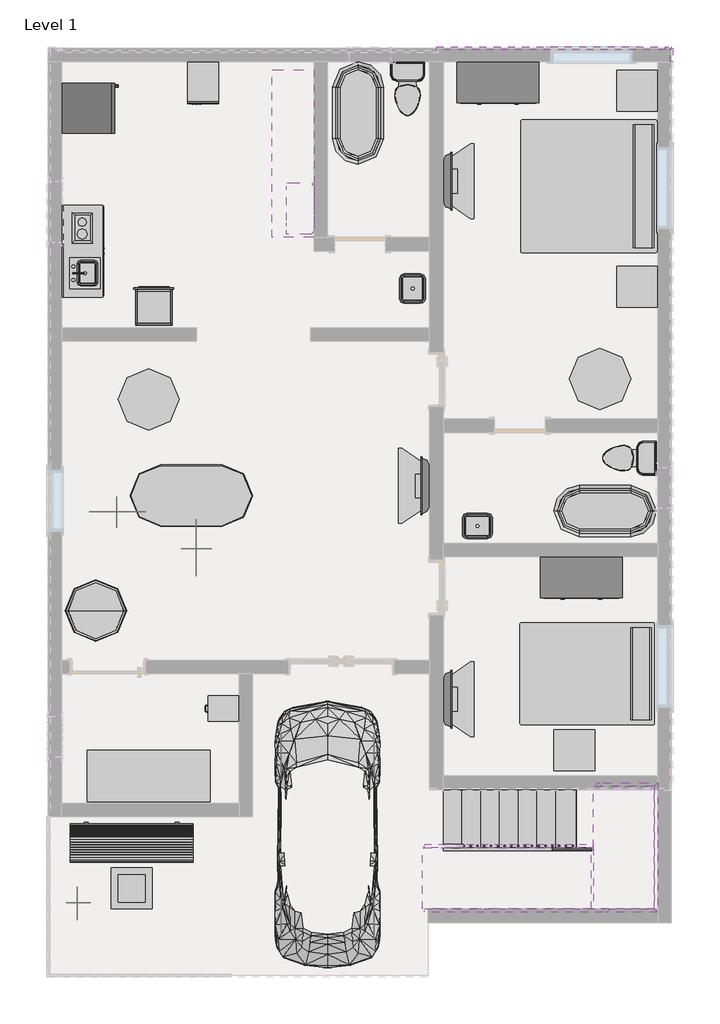
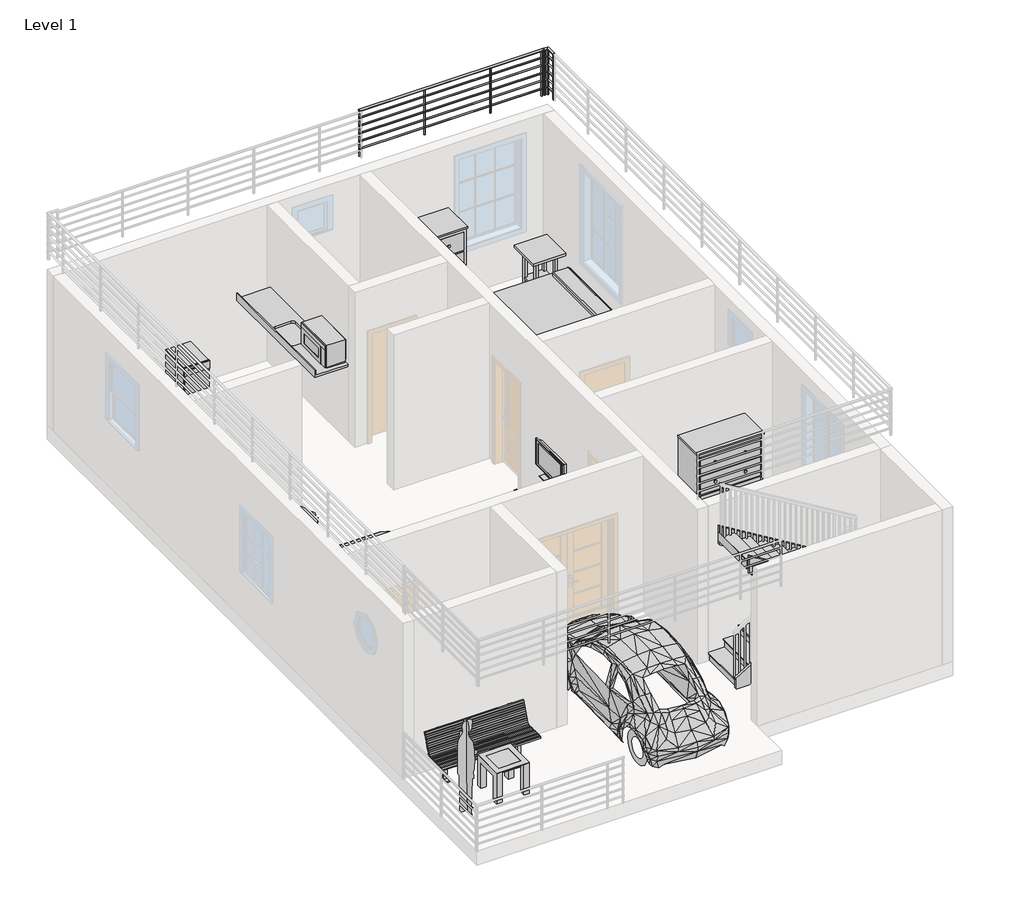
# One storey, part 4 of 4: 22 furniture elements, 10 proxies, 7 flow terminals, 7 members, 3 railings, 2 stair flights, 1 geographic element, 1 slab.
"""IFC4 building model written with IfcOpenShell, lengths in millimetres."""

from ifc_helpers import new_model, si_unit, point, frame, frame_2d, origin, place, context, project, spatial, polyline, circle_curve, trimmed, segment, composite_curve, outline, extrude, faceted_brep, transform, mapped, element, save
from components import proxy_7e1014cc, proxy_fe84b772, proxy_844211aa, proxy_8a8d5ab2, proxy_8b8c2dc4, rpc_beetle_rpc_beetle_3ce7ba48, rpc_female_69e001fa, rpc_male_28878092, proxy_a13a33b2, flow_terminal_871c2e40, flow_terminal_62a433f7, toilet_domestic_3d_toilet_domestic_3d_f7549cf7, toilet_domestic_3d_toilet_domestic_3d_183bbd19, flow_terminal_b374fae2, furniture_1fc5af50, furniture_e1791683, furniture_552c1472, counter_top_w_sink_hole_0600mm_depth_f226a61d, furniture_95afb093, furniture_9fa109b2, furniture_56245f3a, tv_stand_tv_stand_6ce107e5, furniture_b5c51a22, furniture_2c34a4f9, furniture_905aceb5, furniture_4bee3317, furniture_5bc9ed15, furniture_a5b052b6, furniture_c80d6d9c, geographic_element_235d1464, non_monolithic_landing_66cdc52a, stair_flight_35773103, stair_flight_b4d473f5

model = new_model("IFC4")

# Units and contexts
model_context = context("Model", 3, world=origin())
ifc_project = project(units=[si_unit("LENGTHUNIT", "METRE", prefix="MILLI")], contexts=[model_context])

# Site, building, storey
site = spatial("IfcSite", under=ifc_project)
building = spatial("IfcBuilding", under=site)
storey = spatial("IfcBuildingStorey", under=building, Name="Level 1", Elevation=0.0)

# Proxies
placement = place(None, origin())
proxy_shape = proxy_7e1014cc(model_context)
element("IfcBuildingElementProxy", 1, Name="18\" x 24\" x 34 1/2\"", ObjectType="18\" x 24\" x 34 1/2\"", at=placement, inside=storey, context=model_context, shape_type="MappedRepresentation", body=[
    mapped(proxy_shape, transform((-12417.3564253, 14333.684711, 0.0), x_axis=(1.0, 0.0, 0.0), y_axis=(0.0, 1.0, 0.0), z_axis=(0.0, 0.0, 1.0))),
])
proxy_2_shape = proxy_fe84b772(model_context)
element("IfcBuildingElementProxy", 2, Name="Cook Top-2 Unit : 12\" x 18\"", ObjectType="Cook Top-2 Unit : 12\" x 18\"", at=placement, inside=storey, context=model_context, shape_type="MappedRepresentation", body=[
    mapped(proxy_2_shape, transform((-13838.4389568, 12458.6590714, 0.0), x_axis=(-1.0000000000000002, 0.0, 0.0), y_axis=(0.0, -1.0000000000000002, 0.0), z_axis=(0.0, 0.0, 1.0))),
])
proxy_3_shape = proxy_844211aa(model_context)
element("IfcBuildingElementProxy", 3, Name="Kitchenette - Small : 54\"", ObjectType="Kitchenette - Small : 54\"", at=placement, inside=storey, context=model_context, shape_type="MappedRepresentation", body=[
    mapped(proxy_3_shape, transform((-14219.4389568, 12066.7965709, 0.0), x_axis=(0.0, 1.0000000000000002, 0.0), y_axis=(-1.0000000000000002, 0.0, 0.0), z_axis=(0.0, 0.0, 1.0))),
])
proxy_4_shape = proxy_8a8d5ab2(model_context)
element("IfcBuildingElementProxy", 4, Name="Microwave : 30\" x 16\" x 18\"", ObjectType="Microwave : 30\" x 16\" x 18\"", at=placement, inside=storey, context=model_context, shape_type="MappedRepresentation", body=[
    mapped(proxy_4_shape, transform((-10310.358451, 13220.8271532, 609.6), x_axis=(0.0, -1.0000000000000004, 0.0), y_axis=(1.0000000000000004, 0.0, 0.0), z_axis=(0.0, 0.0, 1.0))),
])
proxy_5_shape = proxy_8b8c2dc4(model_context)
element("IfcBuildingElementProxy", 5, Name="Oven Double-Built-in : 21 1/2\" x 39 1/4\" x 21\"", ObjectType="Oven Double-Built-in : 21 1/2\" x 39 1/4\" x 21\"", at=placement, inside=storey, context=model_context, shape_type="MappedRepresentation", body=[
    mapped(proxy_5_shape, transform((-12883.0138841, 11388.4001348, 0.0), x_axis=(-1.0000000000000004, 0.0, 0.0), y_axis=(0.0, -1.0000000000000004, 0.0), z_axis=(0.0, 0.0, 1.0))),
])
rpc_beetle_rpc_beetle_shape = rpc_beetle_rpc_beetle_3ce7ba48(model_context)
element("IfcBuildingElementProxy", 6, Name="RPC Beetle : RPC Beetle", ObjectType="RPC Beetle : RPC Beetle", at=placement, inside=storey, context=model_context, shape_type="MappedRepresentation", body=[
    mapped(rpc_beetle_rpc_beetle_shape, transform((-10257.0389568, 2154.1342758, 0.0), x_axis=(1.0, 0.0, 0.0), y_axis=(0.0, 1.0, 0.0), z_axis=(0.0, 0.0, 1.0))),
])
rpc_female_shape = rpc_female_69e001fa(model_context)
element("IfcBuildingElementProxy", 7, Name="RPC Female", ObjectType="RPC Female", at=placement, inside=storey, context=model_context, shape_type="MappedRepresentation", body=[
    mapped(rpc_female_shape, transform((-13241.5389568, 8191.0885751, 0.0), x_axis=(0.0, 1.0000000000000002, 0.0), y_axis=(-1.0000000000000002, 0.0, 0.0), z_axis=(0.0, 0.0, 1.0))),
])
element("IfcBuildingElementProxy", 8, Name="RPC Female", ObjectType="RPC Female", at=placement, inside=storey, context=model_context, shape_type="MappedRepresentation", body=[
    mapped(rpc_female_shape, transform((-12212.8389568, 7811.9842758, 0.0), x_axis=(-1.0000000000000002, 0.0, 0.0), y_axis=(0.0, -1.0000000000000002, 0.0), z_axis=(0.0, 0.0, 1.0))),
])
rpc_male_shape = rpc_male_28878092(model_context)
element("IfcBuildingElementProxy", 9, Name="RPC Male", ObjectType="RPC Male", at=placement, inside=storey, context=model_context, shape_type="MappedRepresentation", body=[
    mapped(rpc_male_shape, transform((-13990.8389568, 2357.3342758, 0.0), x_axis=(0.0, 1.0000000000000002, 0.0), y_axis=(-1.0000000000000002, 0.0, 0.0), z_axis=(0.0, 0.0, 1.0))),
])
proxy_6_shape = proxy_a13a33b2(model_context)
element("IfcBuildingElementProxy", 10, Name="Refrigerator : 30\" x 32\" RH", ObjectType="Refrigerator : 30\" x 32\" RH", at=placement, inside=storey, context=model_context, shape_type="MappedRepresentation", body=[
    mapped(proxy_6_shape, transform((-13846.3764568, 14211.5853043, 0.0), x_axis=(0.0, 1.0000000000000009, 0.0), y_axis=(-1.0000000000000009, 0.0, 0.0), z_axis=(0.0, 0.0, 1.0))),
])

# Flow terminals
flow_terminal_shape = flow_terminal_871c2e40(model_context)
element("IfcFlowTerminal", 11, ObjectType="Sink Kitchen-Island : 18\" x 18\"", at=placement, inside=storey, context=model_context, shape_type="MappedRepresentation", body=[
    mapped(flow_terminal_shape, transform((-13874.1935557, 11739.6450353, 0.0), x_axis=(0.0, 1.0000000000000002, 0.0), y_axis=(-1.0000000000000002, 0.0, 0.0), z_axis=(0.0, 0.0, 1.0))),
])
flow_terminal_2_shape = flow_terminal_62a433f7(model_context)
element("IfcFlowTerminal", 12, ObjectType="Sink Vanity-Square : 20\" x 18\"", at=placement, inside=storey, context=model_context, shape_type="MappedRepresentation", body=[
    mapped(flow_terminal_2_shape, transform((-8006.1497162, 7934.9796769, 609.6), x_axis=(-1.0000000000000002, 0.0, 0.0), y_axis=(0.0, -1.0000000000000002, 0.0), z_axis=(0.0, 0.0, 1.0))),
])
element("IfcFlowTerminal", 13, ObjectType="Sink Vanity-Square : 20\" x 18\"", at=placement, inside=storey, context=model_context, shape_type="MappedRepresentation", body=[
    mapped(flow_terminal_2_shape, transform((-8938.5843579, 11542.4235164, 609.6), x_axis=(0.0, -1.0, 0.0), y_axis=(1.0, 0.0, 0.0), z_axis=(0.0, 0.0, 1.0))),
])
toilet_domestic_3d_toilet_domestic_3d_shape = toilet_domestic_3d_toilet_domestic_3d_f7549cf7(model_context)
toilet_domestic_3d_toilet_domestic_3d_2_shape = toilet_domestic_3d_toilet_domestic_3d_183bbd19(model_context)
element("IfcFlowTerminal", 14, ObjectType="Toilet-Domestic-3D : Toilet-Domestic-3D", at=placement, inside=storey, context=model_context, shape_type="MappedRepresentation", body=[
    mapped(toilet_domestic_3d_toilet_domestic_3d_shape, transform((-9063.2389568, 14410.2382485, 0.0), x_axis=(1.0000000000000002, 0.0, 0.0), y_axis=(0.0, 1.0000000000000002, 0.0), z_axis=(0.0, 0.0, 1.0))),
    mapped(toilet_domestic_3d_toilet_domestic_3d_2_shape, transform((-9063.2389568, 14410.2382485, 0.0), x_axis=(1.0000000000000002, 0.0, 0.0), y_axis=(0.0, 1.0000000000000002, 0.0), z_axis=(0.0, 0.0, 1.0))),
])
element("IfcFlowTerminal", 15, ObjectType="Toilet-Domestic-3D : Toilet-Domestic-3D", at=placement, inside=storey, context=model_context, shape_type="MappedRepresentation", body=[
    mapped(toilet_domestic_3d_toilet_domestic_3d_shape, transform((-5849.5349842, 8999.4342758, 0.0), x_axis=(0.0, -1.0000000000000004, 0.0), y_axis=(1.0000000000000004, 0.0, 0.0), z_axis=(0.0, 0.0, 1.0))),
    mapped(toilet_domestic_3d_toilet_domestic_3d_2_shape, transform((-5849.5349842, 8999.4342758, 0.0), x_axis=(0.0, -1.0000000000000004, 0.0), y_axis=(1.0000000000000004, 0.0, 0.0), z_axis=(0.0, 0.0, 1.0))),
])
flow_terminal_3_shape = flow_terminal_b374fae2(model_context)
element("IfcFlowTerminal", 16, ObjectType="Tub-Free Standing-3D : 30\" x 60\"", at=placement, inside=storey, context=model_context, shape_type="MappedRepresentation", body=[
    mapped(flow_terminal_3_shape, transform((-9799.8389568, 14142.9342758, 0.0), x_axis=(1.0, 0.0, 0.0), y_axis=(0.0, 1.0, 0.0), z_axis=(0.0, 0.0, 1.0))),
])
element("IfcFlowTerminal", 17, ObjectType="Tub-Free Standing-3D : 30\" x 60\"", at=placement, inside=storey, context=model_context, shape_type="MappedRepresentation", body=[
    mapped(flow_terminal_3_shape, transform((-6116.8389568, 8212.0342758, 0.0), x_axis=(0.0, -1.0000000000000004, 0.0), y_axis=(1.0000000000000004, 0.0, 0.0), z_axis=(0.0, 0.0, 1.0))),
])

# Furniture
furniture_shape = furniture_1fc5af50(model_context)
element("IfcFurniture", 18, ObjectType="Bed-Standard.0001 : King 78\" x 80\"", at=placement, inside=storey, context=model_context, shape_type="MappedRepresentation", body=[
    mapped(furniture_shape, transform((-6312.5438748, 13322.2228004, 0.0), x_axis=(0.0, -1.0, 0.0), y_axis=(1.0, 0.0, 0.0), z_axis=(0.0, 0.0, 1.0))),
])
furniture_2_shape = furniture_e1791683(model_context)
element("IfcFurniture", 19, ObjectType="Bed-Standard.0001 : Queen 60\" x 79\"", at=placement, inside=storey, context=model_context, shape_type="MappedRepresentation", body=[
    mapped(furniture_2_shape, transform((-6337.9438748, 6057.8228004, 0.0), x_axis=(0.0, -1.0, 0.0), y_axis=(1.0, 0.0, 0.0), z_axis=(0.0, 0.0, 1.0))),
])
furniture_3_shape = furniture_552c1472(model_context)
element("IfcFurniture", 20, ObjectType="Cabinet-File 3 Drawer.0001 : 15\" x 18\"", at=placement, inside=storey, context=model_context, shape_type="MappedRepresentation", body=[
    mapped(furniture_3_shape, transform((-11664.3046567, 5137.7378288, 0.0), x_axis=(0.0, -1.0000000000000004, 0.0), y_axis=(1.0000000000000004, 0.0, 0.0), z_axis=(0.0, 0.0, 1.0))),
])
counter_top_w_sink_hole_0600mm_depth_shape = counter_top_w_sink_hole_0600mm_depth_f226a61d(model_context)
element("IfcFurniture", 21, ObjectType="Counter Top w Sink Hole : 0600mm Depth", at=placement, inside=storey, context=model_context, shape_type="MappedRepresentation", body=[
    mapped(counter_top_w_sink_hole_0600mm_depth_shape, transform((-11084.9202068, 13489.1965709, 609.6), x_axis=(0.0, 1.0, 0.0), y_axis=(-1.0, 0.0, 0.0), z_axis=(0.0, 0.0, 1.0))),
])
furniture_4_shape = furniture_95afb093(model_context)
element("IfcFurniture", 22, ObjectType="Counter Top w Sink Hole : 24\" Depth", at=placement, inside=storey, context=model_context, shape_type="MappedRepresentation", body=[
    mapped(furniture_4_shape, transform((-14219.4389568, 12600.1965709, 0.0), x_axis=(0.0, 1.0000000000000002, 0.0), y_axis=(-1.0000000000000002, 0.0, 0.0), z_axis=(0.0, 0.0, 1.0))),
])
furniture_5_shape = furniture_9fa109b2(model_context)
element("IfcFurniture", 23, ObjectType="Dresser : 48\" x 72\" x 24\"", at=placement, inside=storey, context=model_context, shape_type="MappedRepresentation", body=[
    mapped(furniture_5_shape, transform((-7447.845697, 14963.2972299, 0.0), x_axis=(1.0000000000000004, 0.0, 0.0), y_axis=(0.0, 1.0000000000000004, 0.0), z_axis=(0.0, 0.0, 1.0))),
])
element("IfcFurniture", 24, ObjectType="Dresser.0001 : 48\" x 72\" x 24\"", at=placement, inside=storey, context=model_context, shape_type="MappedRepresentation", body=[
    mapped(furniture_5_shape, transform((-6203.245697, 7584.5972299, 0.0), x_axis=(1.0, 0.0, 0.0), y_axis=(0.0, 1.0, 0.0), z_axis=(0.0, 0.0, 1.0))),
])
furniture_6_shape = furniture_56245f3a(model_context)
element("IfcFurniture", 25, ObjectType="TV - Flat Screen : 32\"", at=placement, inside=storey, context=model_context, shape_type="MappedRepresentation", body=[
    mapped(furniture_6_shape, transform((-8471.3003332, 5409.27879, 914.4), x_axis=(0.0, 1.0, 0.0), y_axis=(-1.0, 0.0, 0.0), z_axis=(0.0, 0.0, 1.0))),
])
element("IfcFurniture", 26, ObjectType="TV - Flat Screen : 32\"", at=placement, inside=storey, context=model_context, shape_type="MappedRepresentation", body=[
    mapped(furniture_6_shape, transform((-8471.3003332, 13130.87879, 914.4), x_axis=(0.0, 1.0, 0.0), y_axis=(-1.0, 0.0, 0.0), z_axis=(0.0, 0.0, 1.0))),
])
element("IfcFurniture", 27, ObjectType="TV - Flat Screen : 32\"", at=placement, inside=storey, context=model_context, shape_type="MappedRepresentation", body=[
    mapped(furniture_6_shape, transform((-8797.5381048, 8582.222, 914.4), x_axis=(0.0, -1.0000000000000004, 0.0), y_axis=(1.0000000000000004, 0.0, 0.0), z_axis=(0.0, 0.0, 1.0))),
])
tv_stand_tv_stand_shape = tv_stand_tv_stand_6ce107e5(model_context)
element("IfcFurniture", 28, ObjectType="TV Stand : TV Stand", at=placement, inside=storey, context=model_context, shape_type="MappedRepresentation", body=[
    mapped(tv_stand_tv_stand_shape, transform((-8529.8389568, 13001.7462738, 0.0), x_axis=(0.0, 1.0000000000000002, 0.0), y_axis=(-1.0000000000000002, 0.0, 0.0), z_axis=(0.0, 0.0, 1.0))),
])
element("IfcFurniture", 29, ObjectType="TV Stand : TV Stand", at=placement, inside=storey, context=model_context, shape_type="MappedRepresentation", body=[
    mapped(tv_stand_tv_stand_shape, transform((-8529.8389568, 5280.1462738, 0.0), x_axis=(0.0, 1.0000000000000002, 0.0), y_axis=(-1.0000000000000002, 0.0, 0.0), z_axis=(0.0, 0.0, 1.0))),
])
element("IfcFurniture", 30, ObjectType="TV Stand : TV Stand", at=placement, inside=storey, context=model_context, shape_type="MappedRepresentation", body=[
    mapped(tv_stand_tv_stand_shape, transform((-8738.9994812, 8711.3545162, 0.0), x_axis=(0.0, -1.0000000000000007, 0.0), y_axis=(1.0000000000000007, 0.0, 0.0), z_axis=(0.0, 0.0, 1.0))),
])
furniture_7_shape = furniture_b5c51a22(model_context)
element("IfcFurniture", 31, ObjectType="Table-Coffee : 24\" x 24\" x 24\"", at=placement, inside=storey, context=model_context, shape_type="MappedRepresentation", body=[
    mapped(furniture_7_shape, transform((-13196.3047235, 2490.723198, 0.0), x_axis=(1.0, 0.0, 0.0), y_axis=(0.0, 1.0, 0.0), z_axis=(0.0, 0.0, 1.0))),
])
furniture_8_shape = furniture_2c34a4f9(model_context)
element("IfcFurniture", 32, ObjectType="Table-Dining Oval : 36\" x 72\"", at=placement, inside=storey, context=model_context, shape_type="MappedRepresentation", body=[
    mapped(furniture_8_shape, transform((-12690.8586289, 8082.5359152, 0.0), x_axis=(-1.0, 0.0, 0.0), y_axis=(0.0, -1.0, 0.0), z_axis=(0.0, 0.0, 1.0))),
])
furniture_9_shape = furniture_905aceb5(model_context)
element("IfcFurniture", 33, ObjectType="Table-Dining Round w Chairs : 36\" Diameter", at=placement, inside=storey, context=model_context, shape_type="MappedRepresentation", body=[
    mapped(furniture_9_shape, transform((-13027.720924, 10060.6129644, 0.0), x_axis=(1.0, 0.0, 0.0), y_axis=(0.0, 1.0, 0.0), z_axis=(0.0, 0.0, 1.0))),
])
furniture_10_shape = furniture_4bee3317(model_context)
element("IfcFurniture", 34, ObjectType="Table-Ellipse : 72\" x 36\"", at=placement, inside=storey, context=model_context, shape_type="MappedRepresentation", body=[
    mapped(furniture_10_shape, transform((-6193.0389568, 10180.5342758, 0.0), x_axis=(1.0, 0.0, 0.0), y_axis=(0.0, 1.0, 0.0), z_axis=(0.0, 0.0, 1.0))),
])
furniture_11_shape = furniture_5bc9ed15(model_context)
element("IfcFurniture", 35, ObjectType="Table-Night Stand : 24\" x 24\" x 30\"", at=placement, inside=storey, context=model_context, shape_type="MappedRepresentation", body=[
    mapped(furniture_11_shape, transform((-5942.7725871, 14168.3342758, 0.0), x_axis=(1.0, 0.0, 0.0), y_axis=(0.0, 1.0, 0.0), z_axis=(0.0, 0.0, 1.0))),
])
element("IfcFurniture", 36, ObjectType="Table-Night Stand : 24\" x 24\" x 30\"", at=placement, inside=storey, context=model_context, shape_type="MappedRepresentation", body=[
    mapped(furniture_11_shape, transform((-5942.7725871, 11247.3342758, 0.0), x_axis=(1.0, 0.0, 0.0), y_axis=(0.0, 1.0, 0.0), z_axis=(0.0, 0.0, 1.0))),
])
element("IfcFurniture", 37, ObjectType="Table-Night Stand : 24\" x 24\" x 30\"", at=placement, inside=storey, context=model_context, shape_type="MappedRepresentation", body=[
    mapped(furniture_11_shape, transform((-6882.5725871, 4338.5342758, 0.0), x_axis=(1.0, 0.0, 0.0), y_axis=(0.0, 1.0, 0.0), z_axis=(0.0, 0.0, 1.0))),
])
furniture_12_shape = furniture_a5b052b6(model_context)
element("IfcFurniture", 38, ObjectType="Table-Rectangular : 72\" x 30\"", at=placement, inside=storey, context=model_context, shape_type="MappedRepresentation", body=[
    mapped(furniture_12_shape, transform((-12924.0389568, 4262.3342758, 0.0), x_axis=(1.0, 0.0, 0.0), y_axis=(0.0, 1.0, 0.0), z_axis=(0.0, 0.0, 1.0))),
])
furniture_13_shape = furniture_c80d6d9c(model_context)
element("IfcFurniture", 39, ObjectType="Table-Round : 36\" Diameter", at=placement, inside=storey, context=model_context, shape_type="MappedRepresentation", body=[
    mapped(furniture_13_shape, transform((-13711.4389568, 6726.1342758, 0.0), x_axis=(1.0, 0.0, 0.0), y_axis=(0.0, 1.0, 0.0), z_axis=(0.0, 0.0, 1.0))),
])

# Geographic element
geographic_element_shape = geographic_element_235d1464(model_context)
element("IfcGeographicElement", 40, ObjectType="Park Bench : 72\"", at=placement, inside=storey, context=model_context, shape_type="MappedRepresentation", body=[
    mapped(geographic_element_shape, transform((-13178.0389568, 3297.1342758, 0.0), x_axis=(1.0, 0.0, 0.0), y_axis=(0.0, 1.0, 0.0), z_axis=(0.0, 0.0, 1.0))),
])

# Members
element("IfcMember", 41, ObjectType="Stringer - 2\" Width", at=placement, inside=storey, context=model_context, shape_type="SweptSolid", body=[
    extrude(outline(polyline([(212.114512, -8529.8389568), (0.0, -8529.8389568), (0.0, -8291.753445), (1295.4, -6154.343445), (1600.2, -6239.4979015), (212.114512, -8529.8389568)])), frame((0.0, 4109.9342758, 0.0), z_axis=(0.0, 1.0, 0.0), x_axis=(0.0, 0.0, 1.0)), (0.0, 0.0, 1.0), 50.8),
])
element("IfcMember", 42, ObjectType="Stringer - 2\" Width", at=placement, inside=storey, context=model_context, shape_type="Brep", body=[
    faceted_brep([(-8529.8389568, 3144.7342758, 0.0), (-8529.8389568, 3195.5342758, 0.0), (-8291.753445, 3195.5342758, 0.0), (-8291.753445, 3144.7342758, 0.0), (-8529.8389568, 3144.7342758, 212.114512), (-8529.8389568, 3195.5342758, 212.114512), (-6294.6389568, 3144.7342758, 1566.7811786), (-6294.6389568, 3195.5342758, 1566.7811786), (-6294.6389568, 3195.5342758, 1379.7057504), (-6294.6389568, 3195.5342758, 1210.3724171), (-6294.6389568, 3144.7342758, 1210.3724171)], [[[0, 1, 2, 3]], [[4, 5, 1, 0]], [[5, 4, 6, 7]], [[1, 5, 7, 8, 9, 2]], [[4, 0, 3, 10, 6]], [[2, 9, 10, 3]], [[6, 10, 9, 8, 7]]]),
])
element("IfcMember", 43, ObjectType="Stringer - 2\" Width", at=placement, inside=storey, context=model_context, shape_type="SweptSolid", body=[
    extrude(outline(polyline([(1295.4, -6155.5344686), (1600.2, -6070.3800121), (3260.114512, -8809.2389568), (2903.7057504, -8809.2389568), (1295.4, -6155.5344686)])), frame((0.0, 2230.3342758, 0.0), z_axis=(0.0, 1.0, 0.0), x_axis=(0.0, 0.0, 1.0)), (0.0, 0.0, 1.0), 50.8),
])
element("IfcMember", 44, ObjectType="Stringer - 2\" Width", at=placement, inside=storey, context=model_context, shape_type="Brep", body=[
    faceted_brep([(-8809.2389568, 3246.3342758, 3260.114512), (-8809.2389568, 3246.3342758, 2903.7057504), (-8809.2389568, 3195.5342758, 2903.7057504), (-8809.2389568, 3195.5342758, 3260.114512), (-6294.6389568, 3195.5342758, 1736.114512), (-6294.6389568, 3246.3342758, 1736.114512), (-6294.6389568, 3195.5342758, 1379.7057504), (-6294.6389568, 3195.5342758, 1566.7811786), (-6294.6389568, 3246.3342758, 1379.7057504)], [[[0, 1, 2, 3]], [[4, 5, 0, 3]], [[6, 7, 4, 3, 2]], [[8, 6, 2, 1]], [[5, 8, 1, 0]], [[5, 4, 7, 6, 8]]]),
])
element("IfcMember", 45, ObjectType="Stringer - 2\" Width", at=placement, inside=storey, context=model_context, shape_type="Brep", body=[
    faceted_brep([(-6070.3800121, 2281.1342758, 1600.2), (-6070.3800121, 2230.3342758, 1600.2), (-5329.4389568, 2230.3342758, 1600.2), (-5380.2389568, 2281.1342758, 1600.2), (-6155.5344686, 2281.1342758, 1295.4), (-5380.2389568, 2281.1342758, 1295.4), (-6155.5344686, 2230.3342758, 1295.4), (-5329.4389568, 2230.3342758, 1295.4)], [[[0, 1, 2, 3]], [[4, 0, 3, 5]], [[6, 4, 5, 7]], [[1, 6, 7, 2]], [[1, 0, 4, 6]], [[2, 7, 5, 3]]]),
])
element("IfcMember", 46, ObjectType="Stringer - 2\" Width", at=placement, inside=storey, context=model_context, shape_type="SweptSolid", body=[
    extrude(outline(polyline([(-5329.4389568, 2230.3342758), (-5380.2389568, 2281.1342758), (-5380.2389568, 4109.9342758), (-5329.4389568, 4160.7342758), (-5329.4389568, 2230.3342758)])), frame((0.0, 0.0, 1295.4), z_axis=(0.0, 0.0, 1.0), x_axis=(1.0, 0.0, 0.0)), (0.0, 0.0, 1.0), 304.8),
])
element("IfcMember", 47, ObjectType="Stringer - 2\" Width", at=placement, inside=storey, context=model_context, shape_type="Brep", body=[
    faceted_brep([(-5380.2389568, 4109.9342758, 1600.2), (-5329.4389568, 4160.7342758, 1600.2), (-6239.4979015, 4160.7342758, 1600.2), (-6239.4979015, 4109.9342758, 1600.2), (-5380.2389568, 4109.9342758, 1295.4), (-6154.343445, 4109.9342758, 1295.4), (-5329.4389568, 4160.7342758, 1295.4), (-6154.343445, 4160.7342758, 1295.4)], [[[0, 1, 2, 3]], [[4, 0, 3, 5]], [[6, 4, 5, 7]], [[1, 6, 7, 2]], [[1, 0, 4, 6]], [[2, 7, 5, 3]]]),
])

# Railings
element("IfcRailing", 48, ObjectType="Handrail - Pipe", at=placement, inside=storey, context=model_context, shape_type="SweptSolid", body=[
    extrude(outline(composite_curve([segment(trimmed(circle_curve(frame_2d((4146.55, -5126.2389568)), 19.05), [point((4146.55, -5107.1889568))], [point((4146.55, -5145.2889568))], False, "CARTESIAN"), True, "CONTINUOUS"), segment(trimmed(circle_curve(frame_2d((4146.55, -5126.2389568)), 19.05), [point((4146.55, -5145.2889568))], [point((4146.55, -5107.1889568))], False, "CARTESIAN"), True, "CONTINUOUS")], self_intersect=False)), frame((0.0, 14904.9342758, 0.0), z_axis=(0.0, 1.0, 0.0), x_axis=(0.0, 0.0, 1.0)), (0.0, 0.0, 1.0), 203.2),
    extrude(outline(composite_curve([segment(trimmed(circle_curve(frame_2d((4000.5, -5126.2389568)), 12.7), [point((4000.5, -5138.9389568))], [point((4000.5, -5113.5389568))], False, "CARTESIAN"), True, "CONTINUOUS"), segment(trimmed(circle_curve(frame_2d((4000.5, -5126.2389568)), 12.7), [point((4000.5, -5113.5389568))], [point((4000.5, -5138.9389568))], False, "CARTESIAN"), True, "CONTINUOUS")], self_intersect=False)), frame((0.0, 14904.9342758, 0.0), z_axis=(0.0, 1.0, 0.0), x_axis=(0.0, 0.0, 1.0)), (0.0, 0.0, 1.0), 203.2),
    extrude(outline(composite_curve([segment(trimmed(circle_curve(frame_2d((3848.1, -5126.2389568)), 12.7), [point((3848.1, -5138.9389568))], [point((3848.1, -5113.5389568))], False, "CARTESIAN"), True, "CONTINUOUS"), segment(trimmed(circle_curve(frame_2d((3848.1, -5126.2389568)), 12.7), [point((3848.1, -5113.5389568))], [point((3848.1, -5138.9389568))], False, "CARTESIAN"), True, "CONTINUOUS")], self_intersect=False)), frame((0.0, 14904.9342758, 0.0), z_axis=(0.0, 1.0, 0.0), x_axis=(0.0, 0.0, 1.0)), (0.0, 0.0, 1.0), 203.2),
    extrude(outline(composite_curve([segment(trimmed(circle_curve(frame_2d((3695.7, -5126.2389568)), 12.7), [point((3695.7, -5138.9389568))], [point((3695.7, -5113.5389568))], False, "CARTESIAN"), True, "CONTINUOUS"), segment(trimmed(circle_curve(frame_2d((3695.7, -5126.2389568)), 12.7), [point((3695.7, -5113.5389568))], [point((3695.7, -5138.9389568))], False, "CARTESIAN"), True, "CONTINUOUS")], self_intersect=False)), frame((0.0, 14904.9342758, 0.0), z_axis=(0.0, 1.0, 0.0), x_axis=(0.0, 0.0, 1.0)), (0.0, 0.0, 1.0), 203.2),
    extrude(outline(composite_curve([segment(trimmed(circle_curve(frame_2d((3543.3, -5126.2389568)), 12.7), [point((3543.3, -5138.9389568))], [point((3543.3, -5113.5389568))], False, "CARTESIAN"), True, "CONTINUOUS"), segment(trimmed(circle_curve(frame_2d((3543.3, -5126.2389568)), 12.7), [point((3543.3, -5113.5389568))], [point((3543.3, -5138.9389568))], False, "CARTESIAN"), True, "CONTINUOUS")], self_intersect=False)), frame((0.0, 14904.9342758, 0.0), z_axis=(0.0, 1.0, 0.0), x_axis=(0.0, 0.0, 1.0)), (0.0, 0.0, 1.0), 203.2),
    extrude(outline(composite_curve([segment(trimmed(circle_curve(frame_2d((3390.9, -5126.2389568)), 12.7), [point((3390.9, -5138.9389568))], [point((3390.9, -5113.5389568))], False, "CARTESIAN"), True, "CONTINUOUS"), segment(trimmed(circle_curve(frame_2d((3390.9, -5126.2389568)), 12.7), [point((3390.9, -5113.5389568))], [point((3390.9, -5138.9389568))], False, "CARTESIAN"), True, "CONTINUOUS")], self_intersect=False)), frame((0.0, 14904.9342758, 0.0), z_axis=(0.0, 1.0, 0.0), x_axis=(0.0, 0.0, 1.0)), (0.0, 0.0, 1.0), 203.2),
    extrude(outline(composite_curve([segment(trimmed(circle_curve(frame_2d((-5126.2389568, 15095.4342758)), 12.7), [point((-5138.9389568, 15095.4342758))], [point((-5113.5389568, 15095.4342758))], False, "CARTESIAN"), True, "CONTINUOUS"), segment(trimmed(circle_curve(frame_2d((-5126.2389568, 15095.4342758)), 12.7), [point((-5113.5389568, 15095.4342758))], [point((-5138.9389568, 15095.4342758))], False, "CARTESIAN"), True, "CONTINUOUS")], self_intersect=False)), frame((0.0, 0.0, 3251.2), z_axis=(0.0, 0.0, 1.0), x_axis=(1.0, 0.0, 0.0)), (0.0, 0.0, 1.0), 876.3),
    extrude(outline(composite_curve([segment(trimmed(circle_curve(frame_2d((-5126.2389568, 14917.6342758)), 12.7), [point((-5138.9389568, 14917.6342758))], [point((-5113.5389568, 14917.6342758))], False, "CARTESIAN"), True, "CONTINUOUS"), segment(trimmed(circle_curve(frame_2d((-5126.2389568, 14917.6342758)), 12.7), [point((-5113.5389568, 14917.6342758))], [point((-5138.9389568, 14917.6342758))], False, "CARTESIAN"), True, "CONTINUOUS")], self_intersect=False)), frame((0.0, 0.0, 3251.2), z_axis=(0.0, 0.0, 1.0), x_axis=(1.0, 0.0, 0.0)), (0.0, 0.0, 1.0), 876.3),
])
element("IfcRailing", 49, ObjectType="Handrail - Pipe", at=placement, inside=storey, context=model_context, shape_type="SweptSolid", body=[
    extrude(outline(composite_curve([segment(trimmed(circle_curve(frame_2d((15108.1342758, 4146.55)), 19.05), [point((15089.0842758, 4146.55))], [point((15127.1842758, 4146.55))], False, "CARTESIAN"), True, "CONTINUOUS"), segment(trimmed(circle_curve(frame_2d((15108.1342758, 4146.55)), 19.05), [point((15127.1842758, 4146.55))], [point((15089.0842758, 4146.55))], False, "CARTESIAN"), True, "CONTINUOUS")], self_intersect=False)), frame((-8631.4389568, 0.0, 0.0), z_axis=(1.0, 0.0, 0.0), x_axis=(0.0, 1.0, 0.0)), (0.0, 0.0, 1.0), 3403.6),
    extrude(outline(composite_curve([segment(trimmed(circle_curve(frame_2d((15108.1342758, 4000.5)), 12.7), [point((15120.8342758, 4000.5))], [point((15095.4342758, 4000.5))], False, "CARTESIAN"), True, "CONTINUOUS"), segment(trimmed(circle_curve(frame_2d((15108.1342758, 4000.5)), 12.7), [point((15095.4342758, 4000.5))], [point((15120.8342758, 4000.5))], False, "CARTESIAN"), True, "CONTINUOUS")], self_intersect=False)), frame((-8631.4389568, 0.0, 0.0), z_axis=(1.0, 0.0, 0.0), x_axis=(0.0, 1.0, 0.0)), (0.0, 0.0, 1.0), 3403.6),
    extrude(outline(composite_curve([segment(trimmed(circle_curve(frame_2d((15108.1342758, 3848.1)), 12.7), [point((15120.8342758, 3848.1))], [point((15095.4342758, 3848.1))], False, "CARTESIAN"), True, "CONTINUOUS"), segment(trimmed(circle_curve(frame_2d((15108.1342758, 3848.1)), 12.7), [point((15095.4342758, 3848.1))], [point((15120.8342758, 3848.1))], False, "CARTESIAN"), True, "CONTINUOUS")], self_intersect=False)), frame((-8631.4389568, 0.0, 0.0), z_axis=(1.0, 0.0, 0.0), x_axis=(0.0, 1.0, 0.0)), (0.0, 0.0, 1.0), 3403.6),
    extrude(outline(composite_curve([segment(trimmed(circle_curve(frame_2d((15108.1342758, 3695.7)), 12.7), [point((15120.8342758, 3695.7))], [point((15095.4342758, 3695.7))], False, "CARTESIAN"), True, "CONTINUOUS"), segment(trimmed(circle_curve(frame_2d((15108.1342758, 3695.7)), 12.7), [point((15095.4342758, 3695.7))], [point((15120.8342758, 3695.7))], False, "CARTESIAN"), True, "CONTINUOUS")], self_intersect=False)), frame((-8631.4389568, 0.0, 0.0), z_axis=(1.0, 0.0, 0.0), x_axis=(0.0, 1.0, 0.0)), (0.0, 0.0, 1.0), 3403.6),
    extrude(outline(composite_curve([segment(trimmed(circle_curve(frame_2d((15108.1342758, 3543.3)), 12.7), [point((15120.8342758, 3543.3))], [point((15095.4342758, 3543.3))], False, "CARTESIAN"), True, "CONTINUOUS"), segment(trimmed(circle_curve(frame_2d((15108.1342758, 3543.3)), 12.7), [point((15095.4342758, 3543.3))], [point((15120.8342758, 3543.3))], False, "CARTESIAN"), True, "CONTINUOUS")], self_intersect=False)), frame((-8631.4389568, 0.0, 0.0), z_axis=(1.0, 0.0, 0.0), x_axis=(0.0, 1.0, 0.0)), (0.0, 0.0, 1.0), 3403.6),
    extrude(outline(composite_curve([segment(trimmed(circle_curve(frame_2d((15108.1342758, 3390.9)), 12.7), [point((15120.8342758, 3390.9))], [point((15095.4342758, 3390.9))], False, "CARTESIAN"), True, "CONTINUOUS"), segment(trimmed(circle_curve(frame_2d((15108.1342758, 3390.9)), 12.7), [point((15095.4342758, 3390.9))], [point((15120.8342758, 3390.9))], False, "CARTESIAN"), True, "CONTINUOUS")], self_intersect=False)), frame((-8631.4389568, 0.0, 0.0), z_axis=(1.0, 0.0, 0.0), x_axis=(0.0, 1.0, 0.0)), (0.0, 0.0, 1.0), 3403.6),
    extrude(outline(composite_curve([segment(trimmed(circle_curve(frame_2d((-6193.0389568, 15108.1342758)), 12.7), [point((-6193.0389568, 15120.8342758))], [point((-6193.0389568, 15095.4342758))], False, "CARTESIAN"), True, "CONTINUOUS"), segment(trimmed(circle_curve(frame_2d((-6193.0389568, 15108.1342758)), 12.7), [point((-6193.0389568, 15095.4342758))], [point((-6193.0389568, 15120.8342758))], False, "CARTESIAN"), True, "CONTINUOUS")], self_intersect=False)), frame((0.0, 0.0, 3251.2), z_axis=(0.0, 0.0, 1.0), x_axis=(1.0, 0.0, 0.0)), (0.0, 0.0, 1.0), 876.3),
    extrude(outline(composite_curve([segment(trimmed(circle_curve(frame_2d((-7412.2389568, 15108.1342758)), 12.7), [point((-7412.2389568, 15120.8342758))], [point((-7412.2389568, 15095.4342758))], False, "CARTESIAN"), True, "CONTINUOUS"), segment(trimmed(circle_curve(frame_2d((-7412.2389568, 15108.1342758)), 12.7), [point((-7412.2389568, 15095.4342758))], [point((-7412.2389568, 15120.8342758))], False, "CARTESIAN"), True, "CONTINUOUS")], self_intersect=False)), frame((0.0, 0.0, 3251.2), z_axis=(0.0, 0.0, 1.0), x_axis=(1.0, 0.0, 0.0)), (0.0, 0.0, 1.0), 876.3),
    extrude(outline(composite_curve([segment(trimmed(circle_curve(frame_2d((-5240.5389568, 15108.1342758)), 12.7), [point((-5240.5389568, 15120.8342758))], [point((-5240.5389568, 15095.4342758))], False, "CARTESIAN"), True, "CONTINUOUS"), segment(trimmed(circle_curve(frame_2d((-5240.5389568, 15108.1342758)), 12.7), [point((-5240.5389568, 15095.4342758))], [point((-5240.5389568, 15120.8342758))], False, "CARTESIAN"), True, "CONTINUOUS")], self_intersect=False)), frame((0.0, 0.0, 3251.2), z_axis=(0.0, 0.0, 1.0), x_axis=(1.0, 0.0, 0.0)), (0.0, 0.0, 1.0), 876.3),
    extrude(outline(composite_curve([segment(trimmed(circle_curve(frame_2d((-8618.7389568, 15108.1342758)), 12.7), [point((-8618.7389568, 15120.8342758))], [point((-8618.7389568, 15095.4342758))], False, "CARTESIAN"), True, "CONTINUOUS"), segment(trimmed(circle_curve(frame_2d((-8618.7389568, 15108.1342758)), 12.7), [point((-8618.7389568, 15095.4342758))], [point((-8618.7389568, 15120.8342758))], False, "CARTESIAN"), True, "CONTINUOUS")], self_intersect=False)), frame((0.0, 0.0, 3251.2), z_axis=(0.0, 0.0, 1.0), x_axis=(1.0, 0.0, 0.0)), (0.0, 0.0, 1.0), 876.3),
])
element("IfcRailing", 50, ObjectType="Handrail - Pipe", at=placement, inside=storey, context=model_context, shape_type="SweptSolid", body=[
    extrude(outline(composite_curve([segment(trimmed(circle_curve(frame_2d((15108.1342758, 4146.55)), 19.05), [point((15127.1842758, 4146.55))], [point((15089.0842758, 4146.55))], False, "CARTESIAN"), True, "CONTINUOUS"), segment(trimmed(circle_curve(frame_2d((15108.1342758, 4146.55)), 19.05), [point((15089.0842758, 4146.55))], [point((15127.1842758, 4146.55))], False, "CARTESIAN"), True, "CONTINUOUS")], self_intersect=False)), frame((-5202.4389568, 0.0, 0.0), z_axis=(1.0, 0.0, 0.0), x_axis=(0.0, 1.0, 0.0)), (0.0, 0.0, 1.0), 76.2),
    extrude(outline(composite_curve([segment(trimmed(circle_curve(frame_2d((15108.1342758, 4000.5)), 12.7), [point((15095.4342758, 4000.5))], [point((15120.8342758, 4000.5))], False, "CARTESIAN"), True, "CONTINUOUS"), segment(trimmed(circle_curve(frame_2d((15108.1342758, 4000.5)), 12.7), [point((15120.8342758, 4000.5))], [point((15095.4342758, 4000.5))], False, "CARTESIAN"), True, "CONTINUOUS")], self_intersect=False)), frame((-5202.4389568, 0.0, 0.0), z_axis=(1.0, 0.0, 0.0), x_axis=(0.0, 1.0, 0.0)), (0.0, 0.0, 1.0), 76.2),
    extrude(outline(composite_curve([segment(trimmed(circle_curve(frame_2d((15108.1342758, 3848.1)), 12.7), [point((15095.4342758, 3848.1))], [point((15120.8342758, 3848.1))], False, "CARTESIAN"), True, "CONTINUOUS"), segment(trimmed(circle_curve(frame_2d((15108.1342758, 3848.1)), 12.7), [point((15120.8342758, 3848.1))], [point((15095.4342758, 3848.1))], False, "CARTESIAN"), True, "CONTINUOUS")], self_intersect=False)), frame((-5202.4389568, 0.0, 0.0), z_axis=(1.0, 0.0, 0.0), x_axis=(0.0, 1.0, 0.0)), (0.0, 0.0, 1.0), 76.2),
    extrude(outline(composite_curve([segment(trimmed(circle_curve(frame_2d((15108.1342758, 3695.7)), 12.7), [point((15095.4342758, 3695.7))], [point((15120.8342758, 3695.7))], False, "CARTESIAN"), True, "CONTINUOUS"), segment(trimmed(circle_curve(frame_2d((15108.1342758, 3695.7)), 12.7), [point((15120.8342758, 3695.7))], [point((15095.4342758, 3695.7))], False, "CARTESIAN"), True, "CONTINUOUS")], self_intersect=False)), frame((-5202.4389568, 0.0, 0.0), z_axis=(1.0, 0.0, 0.0), x_axis=(0.0, 1.0, 0.0)), (0.0, 0.0, 1.0), 76.2),
    extrude(outline(composite_curve([segment(trimmed(circle_curve(frame_2d((15108.1342758, 3543.3)), 12.7), [point((15095.4342758, 3543.3))], [point((15120.8342758, 3543.3))], False, "CARTESIAN"), True, "CONTINUOUS"), segment(trimmed(circle_curve(frame_2d((15108.1342758, 3543.3)), 12.7), [point((15120.8342758, 3543.3))], [point((15095.4342758, 3543.3))], False, "CARTESIAN"), True, "CONTINUOUS")], self_intersect=False)), frame((-5202.4389568, 0.0, 0.0), z_axis=(1.0, 0.0, 0.0), x_axis=(0.0, 1.0, 0.0)), (0.0, 0.0, 1.0), 76.2),
    extrude(outline(composite_curve([segment(trimmed(circle_curve(frame_2d((15108.1342758, 3390.9)), 12.7), [point((15095.4342758, 3390.9))], [point((15120.8342758, 3390.9))], False, "CARTESIAN"), True, "CONTINUOUS"), segment(trimmed(circle_curve(frame_2d((15108.1342758, 3390.9)), 12.7), [point((15120.8342758, 3390.9))], [point((15095.4342758, 3390.9))], False, "CARTESIAN"), True, "CONTINUOUS")], self_intersect=False)), frame((-5202.4389568, 0.0, 0.0), z_axis=(1.0, 0.0, 0.0), x_axis=(0.0, 1.0, 0.0)), (0.0, 0.0, 1.0), 76.2),
    extrude(outline(composite_curve([segment(trimmed(circle_curve(frame_2d((-5189.7389568, 15108.1342758)), 12.7), [point((-5189.7389568, 15095.4342758))], [point((-5189.7389568, 15120.8342758))], False, "CARTESIAN"), True, "CONTINUOUS"), segment(trimmed(circle_curve(frame_2d((-5189.7389568, 15108.1342758)), 12.7), [point((-5189.7389568, 15120.8342758))], [point((-5189.7389568, 15095.4342758))], False, "CARTESIAN"), True, "CONTINUOUS")], self_intersect=False)), frame((0.0, 0.0, 3251.2), z_axis=(0.0, 0.0, 1.0), x_axis=(1.0, 0.0, 0.0)), (0.0, 0.0, 1.0), 876.3),
    extrude(outline(composite_curve([segment(trimmed(circle_curve(frame_2d((-5138.9389568, 15108.1342758)), 12.7), [point((-5138.9389568, 15095.4342758))], [point((-5138.9389568, 15120.8342758))], False, "CARTESIAN"), True, "CONTINUOUS"), segment(trimmed(circle_curve(frame_2d((-5138.9389568, 15108.1342758)), 12.7), [point((-5138.9389568, 15120.8342758))], [point((-5138.9389568, 15095.4342758))], False, "CARTESIAN"), True, "CONTINUOUS")], self_intersect=False)), frame((0.0, 0.0, 3251.2), z_axis=(0.0, 0.0, 1.0), x_axis=(1.0, 0.0, 0.0)), (0.0, 0.0, 1.0), 876.3),
])

# Slab
non_monolithic_landing_shape = non_monolithic_landing_66cdc52a(model_context)
element("IfcSlab", 51, ObjectType="Non-Monolithic Landing", at=placement, inside=storey, context=model_context, shape_type="MappedRepresentation", body=[
    mapped(non_monolithic_landing_shape, transform((0.0, 0.0, 0.0), x_axis=(1.0, 0.0, 0.0), y_axis=(0.0, 1.0, 0.0), z_axis=(0.0, 0.0, 1.0))),
])

# Stair flights
stair_flight_shape = stair_flight_35773103(model_context)
element("IfcStairFlight", 52, ObjectType="2\" Tread 1\" Nosing 1/4\" Riser", at=placement, inside=storey, context=model_context, shape_type="MappedRepresentation", body=[
    mapped(stair_flight_shape, transform((0.0, 0.0, 0.0), x_axis=(1.0, 0.0, 0.0), y_axis=(0.0, 1.0, 0.0), z_axis=(0.0, 0.0, 1.0))),
])
stair_flight_2_shape = stair_flight_b4d473f5(model_context)
element("IfcStairFlight", 53, ObjectType="2\" Tread 1\" Nosing 1/4\" Riser", at=placement, inside=storey, context=model_context, shape_type="MappedRepresentation", body=[
    mapped(stair_flight_2_shape, transform((0.0, 0.0, 0.0), x_axis=(1.0, 0.0, 0.0), y_axis=(0.0, 1.0, 0.0), z_axis=(0.0, 0.0, 1.0))),
])

save(model, "model.ifc")

# Revit data of these elements
# Type "18\" x 24\" x 34 1/2\""
#   Label = "T"
#   Assembly Code = "E1090400"
#   Depth = 2' - 0"
#   Height = 2' - 10 1/2"
#   Width = 1' - 6"
#   Panel Face Material = Plastic, Opaque Black
#   Trach Compact. Material = Steel, Paint Finish, Ivory, Matte
#   Default Elevation = 0
# Type "Cook Top-2 Unit : 12\" x 18\""
#   Assembly Code = "E1090400"
#   Counter Height = 3' - 0"
#   Depth = 1' - 6"
#   Width = 1' - 0"
#   Burner Material = Steel, Chrome Plated
#   Cooktop Material = Steel, Polished
#   Default Elevation = 0
# Type "Kitchenette - Small : 54\""
#   Assembly Code = "E1090400"
#   Width = 4' - 6"
#   Height = 2' - 10 1/2"
#   Depth = 2' - 0"
#   Toe Depth = 0' - 3"
#   Toe Height = 0' - 3 1/2"
#   Cabinet Material = Cabinets
#   Door/Drawer Material = Cabinets
#   Handle Material = Cabinets - Handles
#   Default Elevation = 0
# Type "Microwave : 30\" x 16\" x 18\""
#   Assembly Code = "E1090400"
#   Depth = 1' - 4"
#   Height = 1' - 6"
#   Width = 2' - 6"
#   Microwave Material = Laminate, Ivory, Matte
#   Default Elevation = 0
# Type "Oven Double-Built-in : 21 1/2\" x 39 1/4\" x 21\""
#   Label = "OVEN"
#   Assembly Code = "E1090400"
#   Depth = 1' - 9"
#   Height = 3' - 3 1/4"
#   Width = 1' - 9 1/2"
#   Oven Material = Metal - Stainless Steel, Polished
#   Default Elevation = 0
# Type "RPC Beetle : RPC Beetle"
#   built-in parameter 1005195 = "RPC-16-0U6E-L4EG-ENH1-J3KF-SVEL-0TX4-C0"
#   Height = 0
# Type "RPC Female"
#   built-in parameter 1005195 = "RPC-8-FXA2-QQQ0-UGV2-6"
#   Height = 0
# Type "RPC Male"
#   built-in parameter 1005195 = "RPC-8-G1AE-S4G0-CKUK-A"
#   Height = 0
# Type "Refrigerator : 30\" x 32\" RH"
#   Label = "REF."
#   Assembly Code = "E1090400"
#   Depth = 2' - 7 3/4"
#   Handle = 2' - 3"
#   Height = 5' - 10"
#   Rear Clearance = 0' - 2"
#   Top Door Height = 1' - 8"
#   Width = 2' - 5 3/8"
#   Material = Steel, Paint Finish, Ivory, Glossy
#   Default Elevation = 0
# Type "Sink Kitchen-Island : 18\" x 18\""
#   Assembly Code = "D2010410"
#   Counter Height = 3' - 0"
#   Depth = 1' - 6"
#   Width = 1' - 6"
#   Faucet Material = Steel, Polished
#   Sink Material = Steel, Polished
#   Default Elevation = 0
# Type "Sink Vanity-Square : 20\" x 18\""
#   Assembly Code = "D2010400"
#   Counter Height = 2' - 7"
#   Depth = 1' - 6"
#   Width = 1' - 8"
#   Basin Material = Porcelain, Linen
#   Faucet Material = Steel, Polished
#   Default Elevation = 0
# Type "Toilet-Domestic-3D : Toilet-Domestic-3D"
#   Assembly Code = "D2010110"
#   Toilet - Bowl/Basin Material = Porcelain, Linen
#   Toilet - Seat Material = Laminate, Linen, Matte
#   Default Elevation = 0
# Type "Tub-Free Standing-3D : 30\" x 60\""
#   Assembly Code = "D2010110"
#   Height = 1' - 6"
#   Length = 5' - 0"
#   Width = 2' - 6"
#   Tub Material = Porcelain, Ivory
#   Default Elevation = 0
# Type "Bed-Standard.0001 : King 78\" x 80\""
#   Assembly Code = "E2020200"
#   Length = 6' - 8"
#   Width = 6' - 6"
#   Leg Material = Steel, Chrome Plated
#   Mattress Material = Linen, White
#   Default Elevation = 0
# Type "Bed-Standard.0001 : Queen 60\" x 79\""
#   Assembly Code = "E2020200"
#   Length = 6' - 7"
#   Width = 5' - 0"
#   Leg Material = Steel, Chrome Plated
#   Mattress Material = Linen, White
#   Default Elevation = 0
# Type "Cabinet-File 3 Drawer.0001 : 15\" x 18\""
#   Assembly Code = "E2020200"
#   Depth = 1' - 6"
#   Height = 3' - 5"
#   Width = 1' - 3"
#   Cabinet Material = Steel, Paint Finish, Ivory, Glossy
#   Handle Material = Steel, Chrome Plated
#   Default Elevation = 0
# Type "Counter Top w Sink Hole : 0600mm Depth"
#   Assembly Code = "C1030400"
#   Counter Thickness = 0' - 1 9/16"
#   Depth [instance default] = 2' - 0 19/32"
#   Height = 2' - 11 7/16"
#   Length [instance default] = 8' - 2 7/16"
#   Sink Location [instance default] = 3' - 11 1/4"
#   Sink Location To Wall [instance default] = 0' - 3 15/16"
#   Sink Opening Depth [instance default] = 1' - 2 7/8"
#   Sink Opening Width [instance default] = 1' - 11 1/8"
#   Counter Top Material = none
#   Default Elevation = 0
# Type "Counter Top w Sink Hole : 24\" Depth"
#   Assembly Code = "C1030400"
#   Counter Thickness = 0' - 1 1/2"
#   Depth [instance default] = 2' - 1"
#   Height = 3' - 0"
#   Length [instance default] = 8' - 0"
#   Sink Location [instance default] = 2' - 0"
#   Sink Location To Wall [instance default] = 0' - 6"
#   Sink Opening Depth [instance default] = 1' - 3"
#   Sink Opening Width [instance default] = 2' - 3"
#   Counter Top Material = none
#   Default Elevation = 0
# Type "Dresser : 48\" x 72\" x 24\""
#   Assembly Code = "E2020200"
#   Depth = 2' - 0"
#   Height = 6' - 0"
#   Width = 4' - 0"
#   Dresser Material = Laminate - Ivory, Glossy
#   Drawer Material = Laminate, Ivory, Matte
#   Knob Material = Cherry
#   Default Elevation = 0
# Type "Dresser.0001 : 48\" x 72\" x 24\""
#   Assembly Code = "E2020200"
#   Depth = 2' - 0"
#   Height = 6' - 0"
#   Width = 4' - 0"
#   Dresser Material = Laminate - Ivory, Glossy
#   Drawer Material = Laminate, Ivory, Matte
#   Knob Material = Cherry
#   Default Elevation = 0
# Type "TV - Flat Screen : 32\""
#   SinAng = 0' - 0.0193"
#   L = 2' - 3.79372"
#   H = 1' - 3.6354"
#   Thickness = 0' - 4.33071"
#   Diagonal = 2' - 7.88976"
#   CosAng = 0' - 0.03431"
#   Stand [instance default] = yes
#   Default Elevation = 0
# Type "TV Stand : TV Stand"
#   Depth = 1' - 6"
#   Width = 3' - 8"
#   Height = 1' - 7 1/2"
#   Finish = Melamine - Gray
#   Default Elevation = 0
# Type "Table-Coffee : 24\" x 24\" x 24\""
#   Assembly Code = "E2020200"
#   Height = 2' - 0"
#   Length = 2' - 0"
#   Width = 2' - 0"
#   Top Material = none
#   Frame Material = none
#   Default Elevation = 0
# Type "Table-Dining Oval : 36\" x 72\""
#   Assembly Code = "E2020200"
#   Length = 6' - 0"
#   Width = 3' - 0"
#   Base Material = Steel, Chrome Plated
#   Top Material = Glass - Clear, Grey
#   Default Elevation = 0
#   Description = (empty or 0)
# Type "Table-Dining Round w Chairs : 36\" Diameter"
#   Assembly Code = "E2020200"
#   Radius = 1' - 6"
#   Diameter = 3' - 0"
#   Height = 2' - 6"
#   Chairs = 4
#   Base Material = Pine
#   Top Material = Laminate, Linen, Matte
#   Default Elevation = 0
# Type "Table-Ellipse : 72\" x 36\""
#   Assembly Code = "E2020200"
#   Half Width = 1' - 6"
#   Half Length = 1' - 6"
#   Height = 2' - 6"
#   Length = 3' - 0"
#   Width = 3' - 0"
#   Base Material = Birch
#   Top Material = Laminate - Black
#   Default Elevation = 0
# Type "Table-Night Stand : 24\" x 24\" x 30\""
#   Assembly Code = "E2020200"
#   Depth = 2' - 0"
#   Height = 2' - 6"
#   Width = 2' - 0"
#   Base Material = Birch
#   Top Material = Laminate, Ivory, Matte
#   Default Elevation = 0
# Type "Table-Rectangular : 72\" x 30\""
#   Assembly Code = "E2020200"
#   Height = 2' - 6"
#   Length = 6' - 0"
#   Width = 2' - 6"
#   Base Material = Birch
#   Top Material = Birch
#   Default Elevation = 0
# Type "Table-Round : 36\" Diameter"
#   Assembly Code = "E2020200"
#   Base Radius = 0' - 10"
#   Height = 2' - 6"
#   Radius = 1' - 6"
#   Base Material = Steel, Chrome Plated
#   Top Material = Birch
#   Default Elevation = 0
# Type "Park Bench : 72\""
#   Length = 6' - 0"
#   Seat Material = Wood - Teak
#   Frame Material = Steel, Paint Finish, Dark Gray, Matte
# Type "Handrail - Pipe"
#   Assembly Code = "C2010400"
#   built-in parameter 1008612 = 0.0416667 (stored number, unit not read)
#   built-in parameter 1008611 = 0.0833333 (stored number, unit not read)
#   built-in parameter 1008609 = 4 (stored number, unit not read)
#   built-in parameter 1008604 = 0.166667 (stored number, unit not read)
#   built-in parameter 1008603 = 0.166667 (stored number, unit not read)
#   Railing Height = 3' - 0"
#   built-in parameter 1008630 = 2
#   built-in parameter 1008610 = 1
#   built-in parameter 1008605 = 1
#   built-in parameter 1008618 = Baluster - Round : 1"
# Element 1 (IfcBuildingElementProxy, "18\" x 24\" x 34 1/2\"")
#   Phase Created = New Construction
#   Materials on its faces: "Steel, Paint Finish, Ivory, Matte", "Plastic, Opaque Black"
# Element 2 (IfcBuildingElementProxy, "Cook Top-2 Unit : 12\" x 18\"")
#   Phase Created = New Construction
#   Materials on its faces: "Steel, Chrome Plated", "Steel, Polished"
# Element 3 (IfcBuildingElementProxy, "Kitchenette - Small : 54\"")
#   Phase Created = New Construction
#   Materials on its faces: "Cabinets", "Cabinets - Handles"
# Element 4 (IfcBuildingElementProxy, "Microwave : 30\" x 16\" x 18\"")
#   Phase Created = New Construction
#   Materials on its faces: "Laminate, Ivory, Matte", "Glass"
# Element 5 (IfcBuildingElementProxy, "Oven Double-Built-in : 21 1/2\" x 39 1/4\" x 21\"")
#   Phase Created = New Construction
#   Materials on its faces: "Steel", "Metal - Stainless Steel, Polished", "Glass"
# Element 6 (IfcBuildingElementProxy, "RPC Beetle : RPC Beetle")
#   Phase Created = New Construction
# Elements 7, 8 (IfcBuildingElementProxy, "RPC Female")
#   Phase Created = New Construction
# Element 9 (IfcBuildingElementProxy, "RPC Male")
#   Phase Created = New Construction
# Element 10 (IfcBuildingElementProxy, "Refrigerator : 30\" x 32\" RH")
#   Phase Created = New Construction
#   Materials on its faces: "Steel, Paint Finish, Ivory, Glossy", "Steel, Chrome Plated"
# Element 11 (IfcFlowTerminal, "Sink Kitchen-Island : 18\" x 18\"")
#   Mark = "8"
#   Phase Created = New Construction
#   Materials on its faces: "Steel, Polished"
# Element 12 (IfcFlowTerminal, "Sink Vanity-Square : 20\" x 18\"")
#   Mark = "6"
#   Phase Created = New Construction
#   Materials on its faces: "Porcelain, Linen", "Steel, Polished"
# Element 13 (IfcFlowTerminal, "Sink Vanity-Square : 20\" x 18\"")
#   Mark = "7"
#   Phase Created = New Construction
#   Materials on its faces: "Porcelain, Linen", "Steel, Polished"
# Element 14 (IfcFlowTerminal, "Toilet-Domestic-3D : Toilet-Domestic-3D")
#   Mark = "2"
#   Phase Created = New Construction
#   Materials on its faces: "Porcelain, Linen", "Laminate, Linen, Matte"
# Element 15 (IfcFlowTerminal, "Toilet-Domestic-3D : Toilet-Domestic-3D")
#   Mark = "3"
#   Phase Created = New Construction
#   Materials on its faces: "Porcelain, Linen", "Laminate, Linen, Matte"
# Element 16 (IfcFlowTerminal, "Tub-Free Standing-3D : 30\" x 60\"")
#   Mark = "4"
#   Phase Created = New Construction
#   Materials on its faces: "Porcelain, Ivory"
# Element 17 (IfcFlowTerminal, "Tub-Free Standing-3D : 30\" x 60\"")
#   Mark = "5"
#   Phase Created = New Construction
#   Materials on its faces: "Porcelain, Ivory"
# Element 18 (IfcFurniture, "Bed-Standard.0001 : King 78\" x 80\"")
#   Phase Created = New Construction
#   Materials on its faces: "Linen, White", "Steel, Chrome Plated"
# Element 19 (IfcFurniture, "Bed-Standard.0001 : Queen 60\" x 79\"")
#   Phase Created = New Construction
#   Materials on its faces: "Linen, White", "Steel, Chrome Plated"
# Element 20 (IfcFurniture, "Cabinet-File 3 Drawer.0001 : 15\" x 18\"")
#   Phase Created = New Construction
#   Materials on its faces: "Steel, Chrome Plated", "Steel, Paint Finish, Ivory, Glossy"
# Element 21 (IfcFurniture, "Counter Top w Sink Hole : 0600mm Depth")
#   Sink Opening Width = 1' - 11 1/8"
#   Sink Opening Depth = 1' - 2 7/8"
#   Sink Location To Wall = 0' - 3 15/16"
#   Sink Location = 3' - 11 1/4"
#   Length = 8' - 2 7/16"
#   Depth = 2' - 0 19/32"
#   Phase Created = New Construction
#   Materials on its faces: "Counter Top"
# Element 22 (IfcFurniture, "Counter Top w Sink Hole : 24\" Depth")
#   Sink Opening Depth = 1' - 3"
#   Sink Location To Wall = 0' - 6"
#   Length = 4' - 6"
#   Sink Location = 1' - 2"
#   Sink Opening Width = 1' - 4"
#   Depth = 2' - 0"
#   Phase Created = New Construction
#   Materials on its faces: "Counter Top"
# Element 23 (IfcFurniture, "Dresser : 48\" x 72\" x 24\"")
#   Phase Created = New Construction
#   Materials on its faces: "Laminate, Ivory, Matte", "Cherry", "Laminate - Ivory, Glossy"
# Element 24 (IfcFurniture, "Dresser.0001 : 48\" x 72\" x 24\"")
#   Phase Created = New Construction
#   Materials on its faces: "Laminate, Ivory, Matte", "Cherry", "Laminate - Ivory, Glossy"
# Elements 25, 26, 27 (IfcFurniture, "TV - Flat Screen : 32\"")
#   Stand = yes
#   Phase Created = New Construction
#   Materials on its faces: "TV - Black", "TV - Glass", "TV - Screen"
# Elements 28, 29, 30 (IfcFurniture, "TV Stand : TV Stand")
#   Phase Created = New Construction
#   Materials on its faces: "Melamine - Gray", "Glass - Shelves"
# Element 31 (IfcFurniture, "Table-Coffee : 24\" x 24\" x 24\"")
#   Phase Created = New Construction
#   Materials on its faces: "Glass - Clear, Grey"
# Element 32 (IfcFurniture, "Table-Dining Oval : 36\" x 72\"")
#   Phase Created = New Construction
#   Materials on its faces: "Steel, Chrome Plated", "Glass - Clear, Grey"
# Element 33 (IfcFurniture, "Table-Dining Round w Chairs : 36\" Diameter")
#   Phase Created = New Construction
#   Materials on its faces: "Pine", "Laminate, Linen, Matte"
# Element 34 (IfcFurniture, "Table-Ellipse : 72\" x 36\"")
#   Phase Created = New Construction
#   Materials on its faces: "Birch", "Laminate - Black"
# Elements 35, 36, 37 (IfcFurniture, "Table-Night Stand : 24\" x 24\" x 30\"")
#   Phase Created = New Construction
#   Materials on its faces: "Birch", "Laminate, Ivory, Matte"
# Element 38 (IfcFurniture, "Table-Rectangular : 72\" x 30\"")
#   Phase Created = New Construction
#   Materials on its faces: "Birch"
# Element 39 (IfcFurniture, "Table-Round : 36\" Diameter")
#   Phase Created = New Construction
#   Materials on its faces: "Steel, Chrome Plated", "Birch"
# Element 40 (IfcGeographicElement, "Park Bench : 72\"")
#   Phase Created = New Construction
#   Materials on its faces: "Wood - Teak", "Steel, Paint Finish, Dark Gray, Matte"
# Elements 41, 42, 43, 44, 45, 46, 47 (IfcMember, "Stringer - 2\" Width")
#   Phase Created = New Construction
# Elements 48, 49, 50 (IfcRailing, "Handrail - Pipe")
#   built-in parameter 1008621 = 10.6667 (stored number, unit not read)
#   Phase Created = New Construction
# Element 51 (IfcSlab, "Non-Monolithic Landing")
#   Phase Created = New Construction
# Elements 52, 53 (IfcStairFlight, "2\" Tread 1\" Nosing 1/4\" Riser")
#   Phase Created = New Construction
# Materials
#   "Plastic, Opaque Black": class "Plastic", colour RGB 0 0 0, transparency 0.7, Description = "Plastic, generic, opaque black", Cost = 0
#   "Steel, Paint Finish, Ivory, Matte": class "Metal", colour RGB 247 247 239, transparency 0, Description = "Steel, paint finish, ivory, matte", Cost = 0
#   "Steel, Chrome Plated": class "Metal", colour RGB 17 17 17, transparency 0, Description = "Chromiuim plated steel", Cost = 0
#   "Steel, Polished": class "Metal", colour RGB 57 57 57, transparency 0, Description = "Polished steel", Cost = 0
#   "Cabinets": colour RGB 249 249 249, transparency 0
#   "Cabinets - Handles": class "Metal", colour RGB 57 57 57, transparency 0
#   "Laminate, Ivory, Matte": class "Plastic", colour RGB 247 247 239, transparency 0, Description = "Plastic Laminate - Ivory, Matte", Cost = 0
#   "Metal - Stainless Steel, Polished": class "Metal", colour RGB 216 216 216, transparency 0
#   "Steel, Paint Finish, Ivory, Glossy": class "Metal", colour RGB 247 247 239, transparency 0, Description = "Steel, paint finish, ivory, glossy", Cost = 0
#   "Porcelain, Linen": class "Ceramic", colour RGB 249 239 230, transparency 0, Description = "Porcelain, linen", Cost = 0
#   "Laminate, Linen, Matte": class "Plastic", colour RGB 249 239 230, transparency 0, Description = "Plastic Laminate - Linen, Matte", Cost = 0
#   "Porcelain, Ivory": class "Ceramic", colour RGB 247 247 239, transparency 0, Description = "Porcelain, ivory", Cost = 0
#   "Linen, White": class "Textile", colour RGB 247 247 239, transparency 0, Description = "Linen, white", Cost = 0
#   "Laminate - Ivory, Glossy": colour RGB 247 247 239, transparency 0
#   "Cherry": class "Wood", colour RGB 226 177 128, transparency 0, Description = "Prunus Serotina", Cost = 0
#   "Melamine - Gray": class "Wood", colour RGB 49 49 49, transparency 0
#   "Glass - Clear, Grey": class "Glass", colour RGB 252 255 255, transparency 0.64
#   "Pine": class "Wood", colour RGB 223 192 134, transparency 0, Description = "Pinus Echinata", Cost = 0
#   "Birch": class "Wood", colour RGB 210 159 95, transparency 0, Description = "Betula Alleghaniensis", Cost = 0
#   "Laminate - Black": colour RGB 0 0 0, transparency 0
#   "Wood - Teak": class "Wood", colour RGB 120 73 19, transparency 0
#   "Steel, Paint Finish, Dark Gray, Matte": class "Metal", colour RGB 98 98 98, transparency 0, Description = "Steel, paint finish, dark gray, matte", Cost = 0
#   "Glass": class "Glass", colour RGB 0 128 192, transparency 0.75, Description = "Soda Lime Glass", Cost = 0
#   "Steel": class "Metal", colour RGB 247 247 247, transparency 0, Description = "Steel, mill finish", Cost = 0
#   "Counter Top": class "Wood", colour RGB 226 177 128, transparency 0
#   "TV - Black": colour RGB 49 49 49, transparency 0
#   "TV - Glass": colour RGB 157 157 157, transparency 0.9
#   "TV - Screen": colour RGB 0 0 0, transparency 0
#   "Glass - Shelves": class "Glass", colour RGB 167 167 167, transparency 0.9
